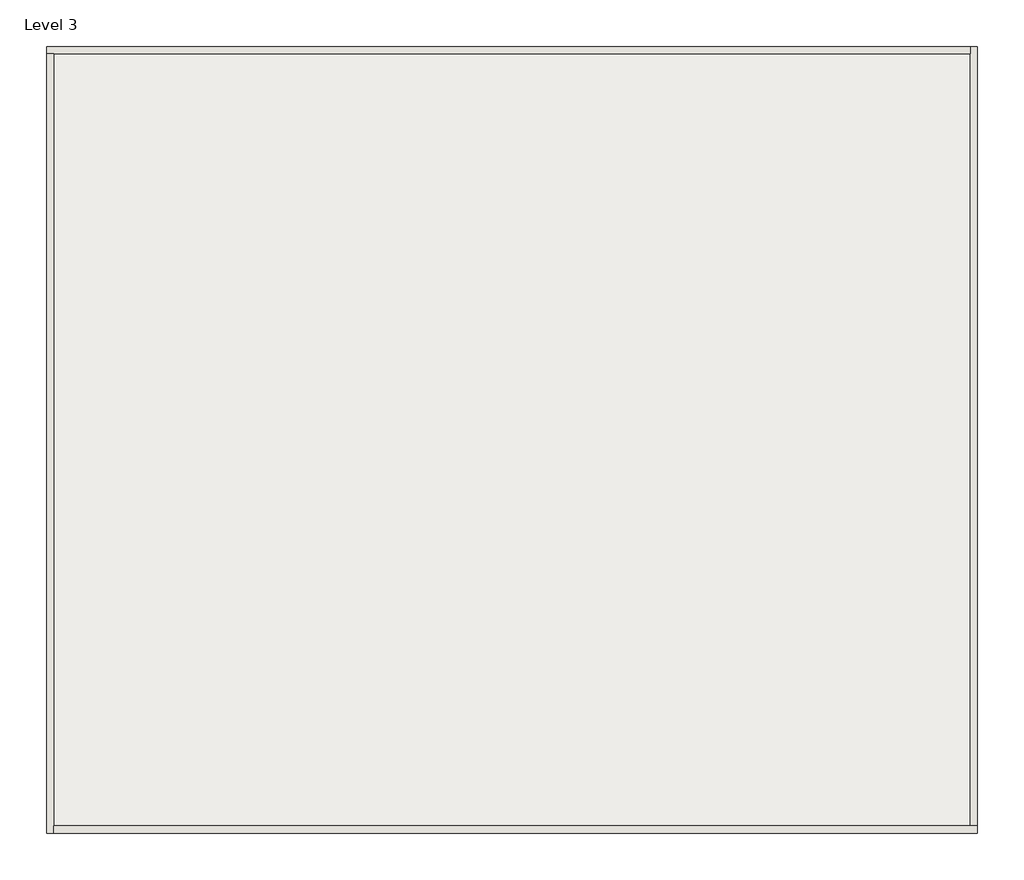
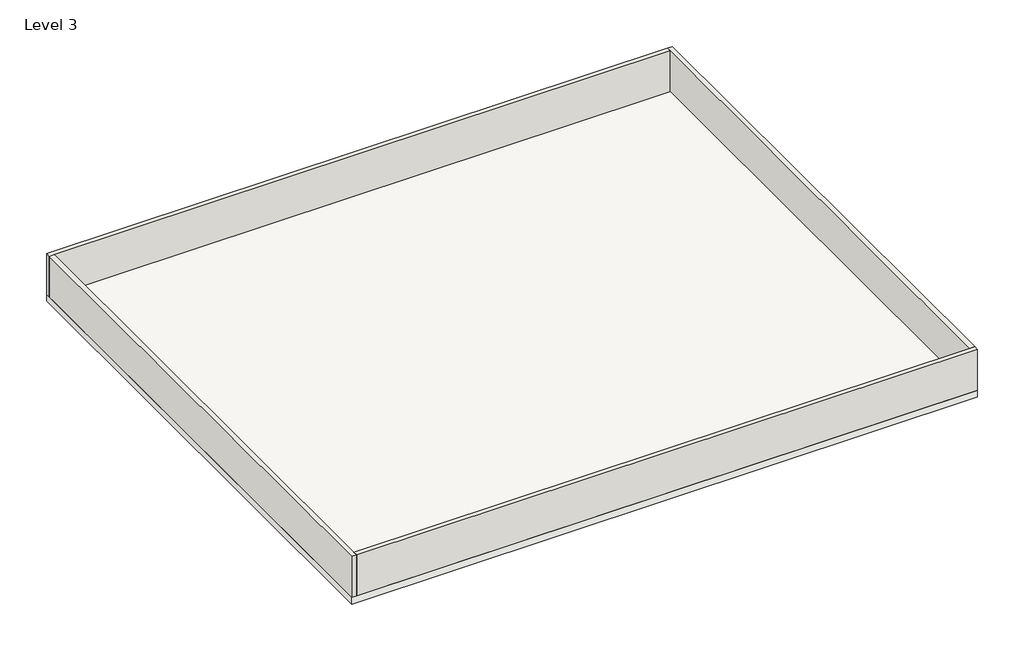
# One storey: 4 walls, 1 slab.
"""IFC4 building model written with IfcOpenShell, lengths in millimetres."""

from ifc_helpers import new_model, si_unit, frame, origin, place, context, project, spatial, polyline, outline, extrude, faceted_brep, element, save

model = new_model("IFC4")

# Units and contexts
model_context = context("Model", 3, world=origin())
ifc_project = project(units=[si_unit("LENGTHUNIT", "METRE", prefix="MILLI")], contexts=[model_context])

# Site, building, storey
site = spatial("IfcSite", under=ifc_project)
building = spatial("IfcBuilding", under=site)
storey = spatial("IfcBuildingStorey", under=building, Name="Level 3", Elevation=6400.8)

# Slab
placement = place(None, origin())
element("IfcSlab", 1, ObjectType="6\"", at=placement, inside=storey, context=model_context, shape_type="SweptSolid", body=[
    extrude(outline(polyline([(831.8132056, 14465.5230289), (831.8132056, 3264.1230289), (-12426.9867944, 3264.1230289), (-12426.9867944, 14465.5230289), (831.8132056, 14465.5230289)])), frame((0.0, 0.0, 6248.4), z_axis=(0.0, 0.0, 1.0), x_axis=(1.0, 0.0, 0.0)), (0.0, 0.0, 1.0), 152.4),
])

# Walls
element("IfcWall", 2, ObjectType="4\"", at=placement, inside=storey, context=model_context, shape_type="Brep", body=[
    faceted_brep([(-12426.9867944, 14363.9230289, 6400.8), (-12325.3867944, 14363.9230289, 6400.8), (730.2132056, 14363.9230289, 6400.8), (730.2132056, 14363.9230289, 7315.2), (-12325.3867944, 14363.9230289, 7315.2), (-12426.9867944, 14363.9230289, 7315.2), (-12426.9867944, 14465.5230289, 6400.8), (-12426.9867944, 14465.5230289, 7315.2), (730.2132056, 14465.5230289, 7315.2), (730.2132056, 14465.5230289, 6400.8)], [[[0, 1, 2, 3, 4, 5]], [[6, 7, 8, 9]], [[2, 1, 0, 6, 9]], [[5, 4, 3, 8, 7]], [[0, 5, 7, 6]], [[3, 2, 9, 8]]]),
])
element("IfcWall", 3, ObjectType="4\"", at=placement, inside=storey, context=model_context, shape_type="Brep", body=[
    faceted_brep([(-12325.3867944, 3264.1230289, 6400.8), (-12325.3867944, 3365.7230289, 6400.8), (-12325.3867944, 14363.9230289, 6400.8), (-12325.3867944, 14363.9230289, 7315.2), (-12325.3867944, 3365.7230289, 7315.2), (-12325.3867944, 3264.1230289, 7315.2), (-12426.9867944, 3264.1230289, 6400.8), (-12426.9867944, 3264.1230289, 7315.2), (-12426.9867944, 14363.9230289, 7315.2), (-12426.9867944, 14363.9230289, 6400.8)], [[[0, 1, 2, 3, 4, 5]], [[6, 7, 8, 9]], [[2, 1, 0, 6, 9]], [[5, 4, 3, 8, 7]], [[0, 5, 7, 6]], [[3, 2, 9, 8]]]),
])
element("IfcWall", 4, ObjectType="4\"", at=placement, inside=storey, context=model_context, shape_type="Brep", body=[
    faceted_brep([(831.8132056, 3365.7230289, 6400.8), (730.2132056, 3365.7230289, 6400.8), (-12325.3867944, 3365.7230289, 6400.8), (-12325.3867944, 3365.7230289, 7315.2), (730.2132056, 3365.7230289, 7315.2), (831.8132056, 3365.7230289, 7315.2), (831.8132056, 3264.1230289, 6400.8), (831.8132056, 3264.1230289, 7315.2), (-12325.3867944, 3264.1230289, 7315.2), (-12325.3867944, 3264.1230289, 6400.8)], [[[0, 1, 2, 3, 4, 5]], [[6, 7, 8, 9]], [[2, 1, 0, 6, 9]], [[5, 4, 3, 8, 7]], [[0, 5, 7, 6]], [[3, 2, 9, 8]]]),
])
element("IfcWall", 5, ObjectType="4\"", at=placement, inside=storey, context=model_context, shape_type="Brep", body=[
    faceted_brep([(730.2132056, 14465.5230289, 6400.8), (730.2132056, 14363.9230289, 6400.8), (730.2132056, 3365.7230289, 6400.8), (730.2132056, 3365.7230289, 7315.2), (730.2132056, 14363.9230289, 7315.2), (730.2132056, 14465.5230289, 7315.2), (831.8132056, 14465.5230289, 6400.8), (831.8132056, 14465.5230289, 7315.2), (831.8132056, 3365.7230289, 7315.2), (831.8132056, 3365.7230289, 6400.8)], [[[0, 1, 2, 3, 4, 5]], [[6, 7, 8, 9]], [[2, 1, 0, 6, 9]], [[5, 4, 3, 8, 7]], [[0, 5, 7, 6]], [[3, 2, 9, 8]]]),
])

save(model, "model.ifc")

# Revit data of these elements
# Type "6\""
#   Assembly Code = "B1010"
#   Function = 0
#   Layers, outside or top first: 0' - 6" "flooring" (function 1)
# Type "4\""
#   Assembly Code = "B2010"
#   Layers, outside or top first: 0' - 4" "EXT WALL" (function 1)
# Element 1 (IfcSlab, "6\"")
#   Height Offset From Level = 0' - 0"
#   Phase Created = New Construction
#   Materials on its faces: "flooring"
# Elements 2, 3, 4, 5 (IfcWall, "4\"")
#   Top Offset = 0' - 0"
#   Base Offset = 0' - 0"
#   Unconnected Height = 3' - 0"
#   wall height = 3' - 0"
#   Phase Created = New Construction
#   Base Constraint = Level 3
#   Materials on its faces: "EXT WALL"
# Materials
#   "flooring": class "Generic", colour RGB 120 120 120, transparency 0, Cost = 0
#   "EXT WALL": class "Generic", colour RGB 159 125 47, transparency 0, Cost = 0
